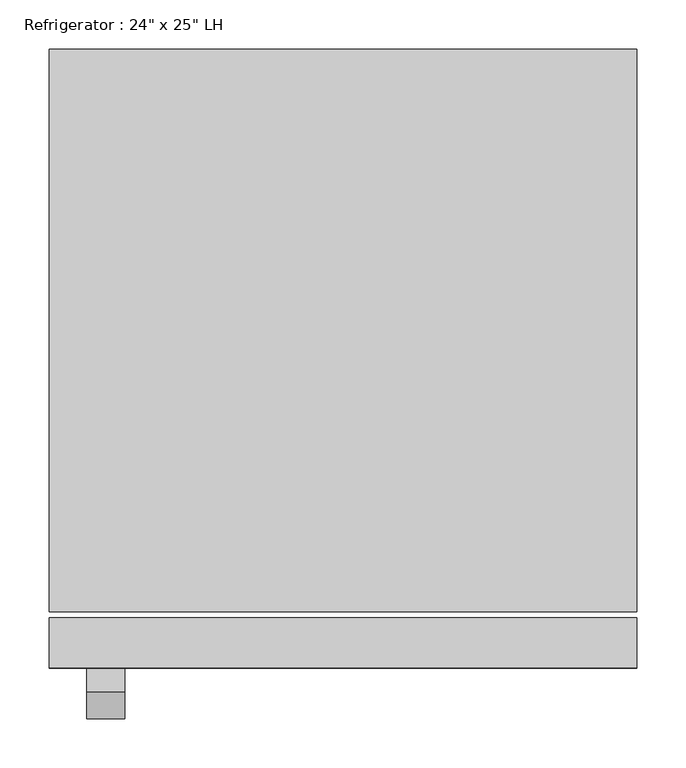
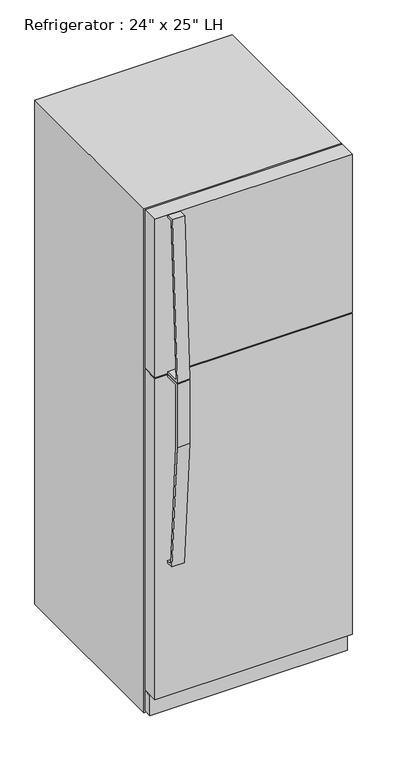
"""IFC4 building model written with IfcOpenShell, lengths in millimetres: proxy geometry."""

from ifc_helpers import new_model, si_unit, frame, origin, origin_with_axes, place, context, project, spatial, polyline, outline, extrude, source, transform, mapped, element, save


def proxy_c523a7b7(model_context):
    return source(origin(), model_context, "Body", "SweptSolid", [
        extrude(outline(polyline([(-329.0010285, 1096.9625), (-373.4510285, 1096.9625), (-373.4510285, 900.3342469), (-345.9723987, 507.3715334), (-329.0010285, 507.3715334), (-329.0010285, 501.0370017), (-351.8949512, 501.0370017), (-379.8010285, 900.1125), (-379.8010285, 1103.3125), (-329.0010285, 1103.3125), (-329.0010285, 1096.9625)])), frame((-260.35, 0.0, 0.0), z_axis=(1.0, 0.0, 0.0), x_axis=(0.0, 1.0, 0.0)), (0.0, 0.0, 1.0), 38.4332978),
        extrude(outline(polyline([(-353.839413, 1612.9), (-329.7780855, 1612.9), (-329.7780855, 1606.55), (-348.6263449, 1606.55), (-374.5007207, 1112.8375), (-329.7780855, 1112.8375), (-329.7780855, 1106.4875), (-380.3793675, 1106.4875), (-353.839413, 1612.9)])), frame((-260.35, 0.0, 0.0), z_axis=(1.0, 0.0, 0.0), x_axis=(0.0, 1.0, 0.0)), (0.0, 0.0, 1.0), 38.4332978),
        extrude(outline(polyline([(298.45, -278.2010285), (298.45, -303.6010285), (-298.45, -303.6010285), (-298.45, -278.2010285), (298.45, -278.2010285)])), frame((0.0, 0.0, 9.3816357), z_axis=(0.0, 0.0, 1.0), x_axis=(1.0, 0.0, 0.0)), (0.0, 0.0, 1.0), 63.5),
        extrude(outline(polyline([(298.45, -278.2010285), (298.45, -329.0010285), (-298.45, -329.0010285), (-298.45, -278.2010285), (298.45, -278.2010285)])), frame((0.0, 0.0, 76.2), z_axis=(0.0, 0.0, 1.0), x_axis=(1.0, 0.0, 0.0)), (0.0, 0.0, 1.0), 1027.1125),
        extrude(outline(polyline([(298.45, -278.2010285), (298.45, -329.0010285), (-298.45, -329.0010285), (-298.45, -278.2010285), (298.45, -278.2010285)])), frame((0.0, 0.0, 1106.4875), z_axis=(0.0, 0.0, 1.0), x_axis=(1.0, 0.0, 0.0)), (0.0, 0.0, 1.0), 506.4125),
        extrude(outline(polyline([(298.45, 299.6489715), (298.45, -271.8510285), (-298.45, -271.8510285), (-298.45, 299.6489715), (298.45, 299.6489715)])), origin_with_axes(), (0.0, 0.0, 1.0), 1612.9),
    ])


if __name__ == "__main__":
    model = new_model("IFC4")
    model_context = context("Model", 3, world=origin())
    ifc_project = project(units=[si_unit("LENGTHUNIT", "METRE", prefix="MILLI")], contexts=[model_context])
    site = spatial("IfcSite", under=ifc_project)
    building = spatial("IfcBuilding", under=site)
    placement = place(None, origin())
    proxy_shape = proxy_c523a7b7(model_context)
    element("IfcBuildingElementProxy", 1, Name="Refrigerator : 24\" x 25\" LH", ObjectType="Refrigerator : 24\" x 25\" LH", at=placement, inside=building, context=model_context, shape_type="MappedRepresentation", body=[
        mapped(proxy_shape, transform((0.0, 0.0, 0.0), x_axis=(1.0, 0.0, 0.0), y_axis=(0.0, 1.0, 0.0), z_axis=(0.0, 0.0, 1.0))),
    ])
    save(model, "model.ifc")

# Revit data of these elements
# Type "Refrigerator : 24\" x 25\" LH"
#   Label = "REF."
#   Assembly Code = "E1090400"
#   Depth = 2' - 0 3/4"
#   Handle = 0' - 1 1/2"
#   Height = 5' - 3 1/2"
#   Rear Clearance = 0' - 2"
#   Top Door Height = 1' - 8"
#   Width = 1' - 11 1/2"
#   Material = Steel, Paint Finish, Ivory, Glossy
#   Default Elevation = 0
# Element 1 (IfcBuildingElementProxy, "Refrigerator : 24\" x 25\" LH")
#   Materials on its faces: "Steel, Paint Finish, Ivory, Glossy", "Steel, Chrome Plated"
# Materials
#   "Steel, Paint Finish, Ivory, Glossy": class "Metal", colour RGB 247 247 239, transparency 0, Description = "Steel, paint finish, ivory, glossy", Cost = 0
#   "Steel, Chrome Plated": class "Metal", colour RGB 216 216 216, transparency 0, Description = "Chromiuim plated steel", Cost = 0
